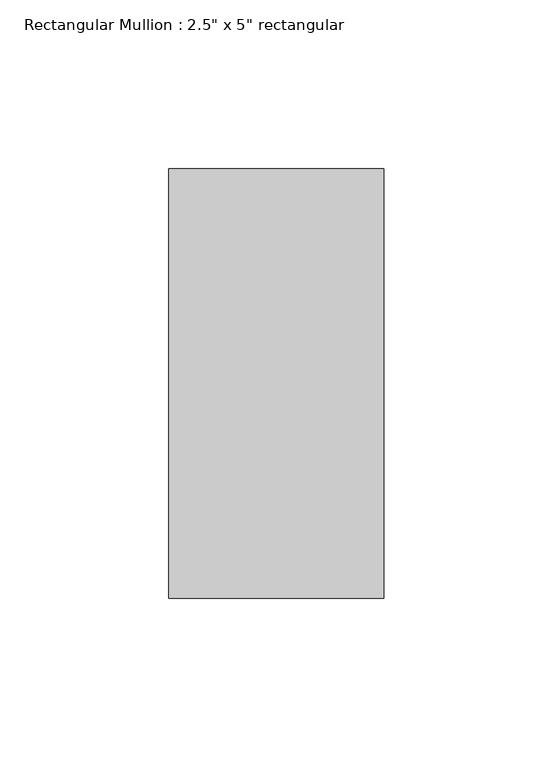
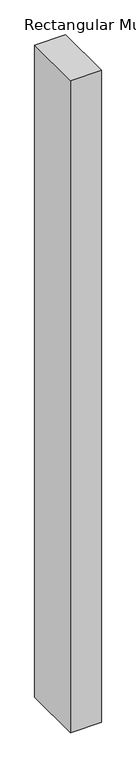
"""IFC4 building model written with IfcOpenShell, lengths in millimetres: member geometry."""

from ifc_helpers import new_model, si_unit, frame, origin, place, context, project, spatial, polyline, outline, extrude, source, transform, mapped, element, save


def member_7354043d(model_context):
    return source(origin(), model_context, "Body", "SweptSolid", [
        extrude(outline(polyline([(31.75, 63.5), (31.75, -63.5), (-31.75, -63.5), (-31.75, 63.5), (31.75, 63.5)])), frame((0.0, 0.0, -1416.05), z_axis=(0.0, 0.0, 1.0), x_axis=(1.0, 0.0, 0.0)), (0.0, 0.0, 1.0), 1416.05),
    ])


if __name__ == "__main__":
    model = new_model("IFC4")
    model_context = context("Model", 3, world=origin())
    ifc_project = project(units=[si_unit("LENGTHUNIT", "METRE", prefix="MILLI")], contexts=[model_context])
    site = spatial("IfcSite", under=ifc_project)
    building = spatial("IfcBuilding", under=site)
    placement = place(None, origin())
    member_shape = member_7354043d(model_context)
    element("IfcMember", 1, ObjectType="Rectangular Mullion : 2.5\" x 5\" rectangular", at=placement, inside=building, context=model_context, shape_type="MappedRepresentation", body=[
        mapped(member_shape, transform((0.0, 0.0, 0.0), x_axis=(1.0, 0.0, 0.0), y_axis=(0.0, 1.0, 0.0), z_axis=(0.0, 0.0, 1.0))),
    ])
    save(model, "model.ifc")

# Revit data of these elements
# Type "Rectangular Mullion : 2.5\" x 5\" rectangular"
#   built-in parameter 1007304 = 0.416667 (stored number, unit not read)
#   built-in parameter 1007301 = 0.104167 (stored number, unit not read)
#   built-in parameter 1007300 = 0.104167 (stored number, unit not read)
# Element 1 (IfcMember, "Rectangular Mullion : 2.5\" x 5\" rectangular")
#   Materials on its faces: "Aluminum"
# Materials
#   "Aluminum": class "Metal", colour RGB 247 247 247, transparency 0, Description = "Aluminum 6061", Cost = 0
